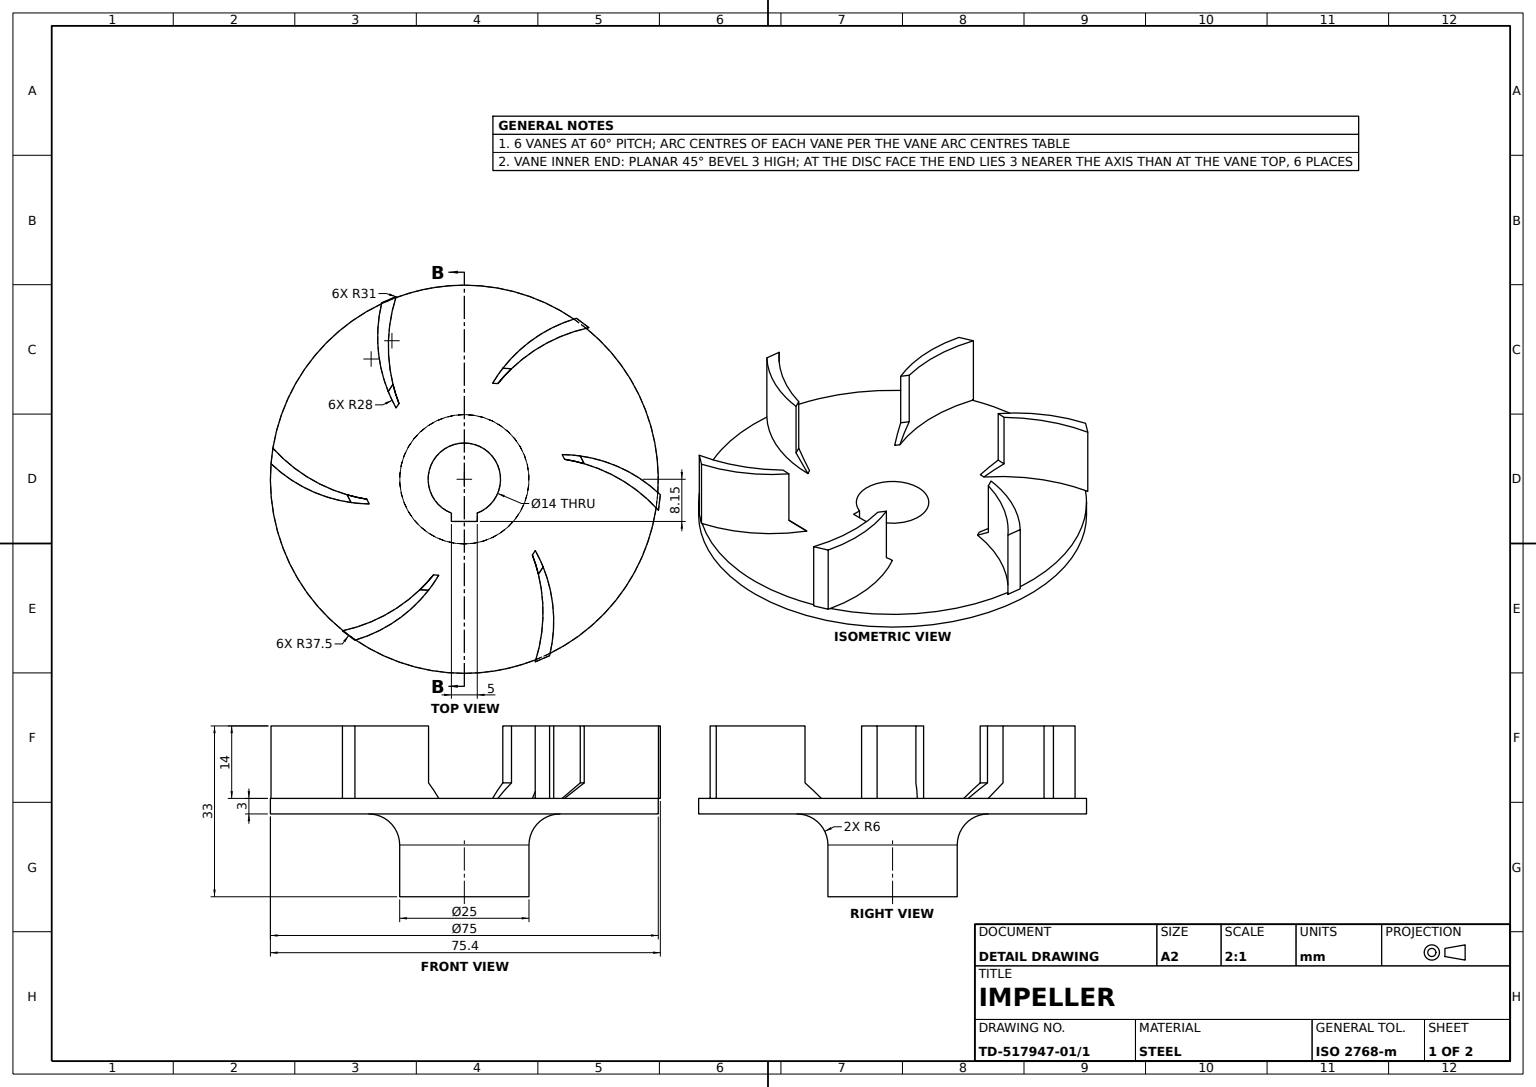
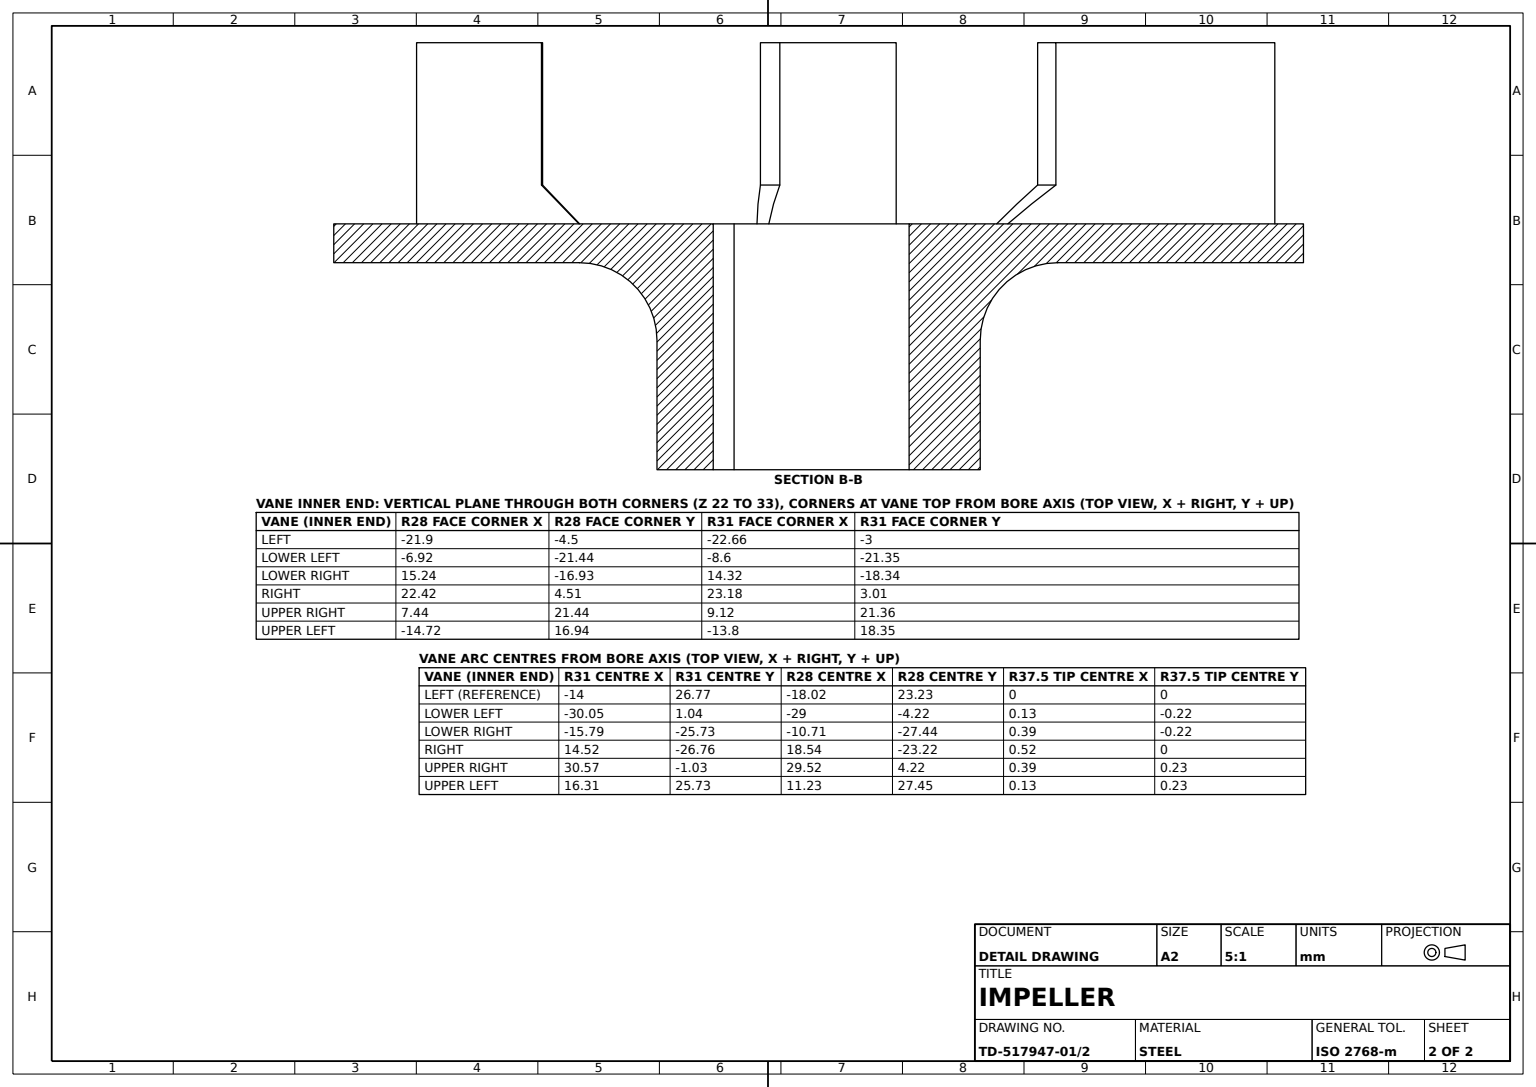
from build123d import *
from build123d.topology import SkipClean

# Parameters (mm, degrees)
BASE_DISC_SKETCH_R                         = 37.5
BASE_DISC_75_DEPTH                         = 3
VANE_DEPTH                                 = 14
VANE_CHAMFER_3MM_SIZE                      = 3
VANE_PATTERN_6X60_COUNT                    = 6
VANE_CHAMFER_3MM_OF_VANE_PATTERN_6X60_SIZE = 3
HUB_SKETCH_R                               = 12.5
HUB_25_DEPTH                               = 16
SHAFT_BORE_14_DEPTH                        = 63.702444686
SHAFT_BORE_14_DEPTH_BACK                   = 63.702444686
HUB_FILLET_R6_R                            = 6


with BuildPart() as part:
    # Base Disc Sketch → Base Disc Ø75 (new body)
    with BuildSketch(Plane(origin=(0, 0, 0), x_dir=(1, 0, 0), z_dir=(0, 1, 0))):
        with Locations(Location((0, 0, 0), (0, 0, 270))):
            Circle(BASE_DISC_SKETCH_R)
    extrude(amount=BASE_DISC_75_DEPTH)

    # Vane Profile Sketch → Vane (add)
    with SkipClean():  # the faces are left unmerged after this step: merging them gives an invalid solid
        with BuildSketch(Plane(origin=(0, 3, 0), x_dir=(1, 0, 0), z_dir=(0, 1, 0))):
            with BuildLine():
                Line((-22.661730354, -3), (-21.896634912, -4.5))
                ThreePointArc((-21.896634912, -4.5), (-30.228522345, -1.968631367), (-37.379807383, 3))
                ThreePointArc((-37.379807383, 3), (-37.228578705, 4.503657138), (-37.016888038, 6))
                ThreePointArc((-37.016888038, 6), (-30.466111276, 0.5002397), (-22.661730354, -3))
            make_face()
        vane = extrude(amount=VANE_DEPTH)

    # Vane Chamfer 3mm
    vane_chamfer_3mm_edges = [part.edges().sort_by_distance(p)[0] for p in [
        (-22.279182633, 3, 3.75),
    ]]
    chamfer(vane_chamfer_3mm_edges, length=VANE_CHAMFER_3MM_SIZE)

    # Vane Pattern 6x60°: Vane ×6 about axis
    with SkipClean():  # the faces are left unmerged after this step: merging them gives an invalid solid
        vane_pattern_6x60_axis = Axis((0.259677898, 0, -0.003858097), (0, 1, 0))
        for i in range(1, VANE_PATTERN_6X60_COUNT):
            add(vane.rotate(vane_pattern_6x60_axis, i * 360 / VANE_PATTERN_6X60_COUNT))

    # Vane Chamfer 3mm of Vane Pattern 6x60°
    vane_chamfer_3mm_of_vane_pattern_6x60_edges = [part.edges().sort_by_distance(p)[0] for p in [
        (-7.758815893, 3, 21.392296743),
        (14.780044637, 3, 17.638438646),
        (22.798538428, 3, -3.757716194),
        (8.278171688, 3, -21.400012937),
        (-14.260688842, 3, -17.64615484),
    ]]
    chamfer(vane_chamfer_3mm_of_vane_pattern_6x60_edges, length=VANE_CHAMFER_3MM_OF_VANE_PATTERN_6X60_SIZE)

    # Hub Sketch → Hub Ø25 (add)
    with SkipClean():  # the faces are left unmerged after this step: merging them gives an invalid solid
        with BuildSketch(Plane.XZ):
            with Locations(Location((0, 0, 0), (0, 0, 270))):
                Circle(HUB_SKETCH_R)
        extrude(amount=HUB_25_DEPTH)

    # Shaft Bore Sketch → Shaft Bore Ø14 (cut, two sides: drawn at the far end of the back side and taken through both)
    with SkipClean():  # the faces are left unmerged after this step: merging them gives an invalid solid
        with BuildSketch(Plane.XZ.offset(16).offset(-SHAFT_BORE_14_DEPTH_BACK)):
            with BuildLine():
                Line((-2.5, 8.15), (2.5, 8.15))
                Line((2.5, 8.15), (2.5, 6.538348415))
                ThreePointArc((2.5, 6.538348415), (0, -7), (-2.5, 6.538348415))
                Line((-2.5, 6.538348415), (-2.5, 8.15))
            make_face()
        extrude(amount=SHAFT_BORE_14_DEPTH + SHAFT_BORE_14_DEPTH_BACK, mode=Mode.SUBTRACT)

    # Hub Fillet R6
    hub_fillet_r6_edges = [part.edges().sort_by_distance(p)[0] for p in [
        (0, 0, 12.5),
    ]]
    fillet(hub_fillet_r6_edges, radius=HUB_FILLET_R6_R)


solid = part.part
